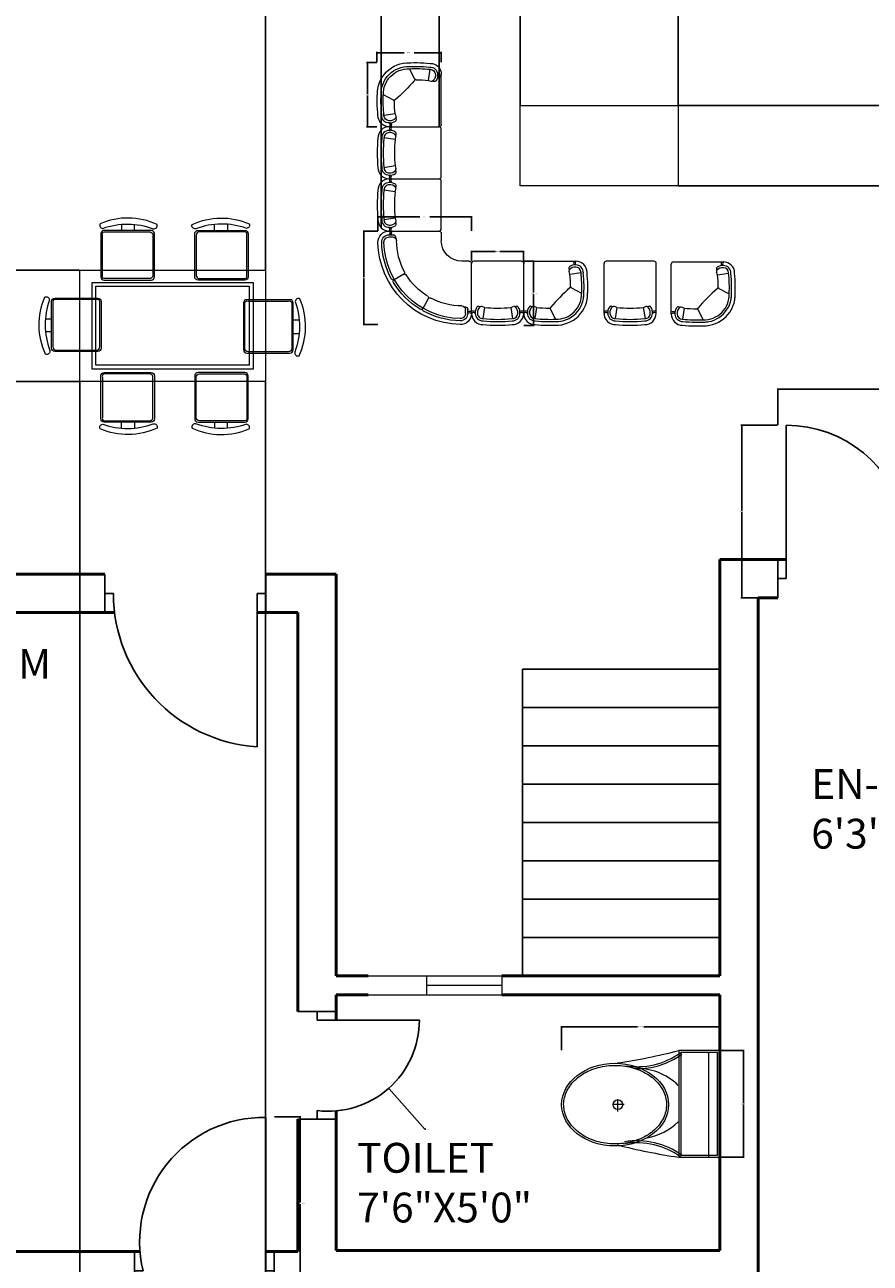
# Model space of a CAD drawing. Units: inches. Extents: x 2215 to 3724, y 1009 to 2124.
# Tile 3 of 11: x 2438 to 2636, y 1158 to 1449. Entities that reach past the tile are written whole.
import ezdxf

# ---------------------------------------------------------------- set-up
doc = ezdxf.new("R2010")
doc.units = ezdxf.units.IN
for name, color, linetype, lineweight in [('A-ANNO-DIMS', 2, 'Continuous', 18), ('A-AREA-IDEN', 7, 'Continuous', 18), ('A-DOOR', 3, 'Continuous', 25), ('A-FLOR-FIXT', 9, 'Continuous', 18), ('A-FLOR-STRS', 7, 'Continuous', 25), ('A-FURN', 8, 'Continuous', 18), ('A-GLAZ', 4, 'Continuous', 18), ('A-WALL', 7, 'Continuous', 50)]:
    doc.layers.add(name, color=color, linetype=linetype, lineweight=lineweight)
doc.styles.get("Standard").update_dxf_attribs({"font": 'arial.ttf'})
doc.dimstyles.get("Standard").update_dxf_attribs({"dimtxt": 0.18, "dimasz": 0.18, "dimexe": 0.18, "dimexo": 0.0625, "dimgap": 0.09, "dimtad": 0, "dimtih": 1, "dimtoh": 1, "dimdec": 4, "dimzin": 0, "dimdsep": 46, "dimtxsty": 'Standard', "dimcen": 0.09, "dimadec": 0, "dimazin": 0, "dimtfac": 1, "dimtdec": 4, "dimtofl": 0, "dimtmove": 0, "dimatfit": 3, "dimfxl": 1, "dimtolj": 1, "dimtzin": 0, "dimarcsym": 0})

# ---------------------------------------------------------------- blocks, each defined once
blk = doc.blocks.new('A$C31115884')
for p, q in [((283.1, 497.7), (223.4, 497.7)), ((257.5, 466.4), (257.5, 523.2)), ((0, 200), (0, 0)), ((520, 200), (0, 200)), ((10, 190), (10, 10)), ((510, 190), (10, 190)), ((510, 10), (510, 190)), ((520, 0), (520, 200)), ((510, 54.5), (0, 54.5)), ((10, 10), (510, 10)), ((0, 0), (520, 0))]:
    blk.add_line(p, q)
blk.add_circle((255.6, 496.4), 23.6)
for centre, radius, start, end in [((2777.7, -204.6), 2807, 165.4549, 171.71327), ((3237, 905), 2807, 188.28673, 194.5451), ((-294.5, 403.3), 364.7, 324.20913, 9.34987), ((-294.5, 403.3), 374.7, 324.20913, 9.34987), ((805.8, 403.3), 364.7, 170.65013, 215.79087), ((139.5, 406.2), 293.5, 315.84364, 2.65635), ((805.8, 403.3), 374.7, 179.20365, 215.79087), ((383.6, 406.2), 293.5, 190.27735, 224.15636)]:
    blk.add_arc(centre, radius, start, end)
blk.add_ellipse((256.2, 509.9), major_axis=(0, -260.7), ratio=0.772727)
blk.add_open_spline([(256.2, 259.2), (263.1, 259.2), (270, 259.7), (287.8, 262.3), (298.7, 265.1), (319.9, 273.1), (330.2, 278.4), (350.1, 291.1), (359.7, 298.7), (377.7, 315.9), (386.2, 325.5), (401.7, 346.6), (408.8, 358.1), (421.3, 382.5), (426.8, 395.5), (435.9, 422.4), (439.5, 436.4), (444.8, 465.1), (446.5, 479.7), (447.9, 509.2), (447.6, 524), (445, 553.3), (442.7, 567.8), (436.3, 596), (432.1, 609.7), (421.9, 636), (416, 648.6), (402.5, 672.1), (395, 683), (378.6, 703), (369.8, 712.1), (351.1, 728), (341.3, 734.8), (320.9, 746.2), (310.4, 750.7), (288.9, 757.3), (278, 759.4), (256, 761), (245, 760.6), (223.1, 757.2), (212.3, 754.3), (191.1, 746.1), (180.8, 740.7), (160.9, 727.8), (151.4, 720.1), (133.5, 702.7), (125.1, 693), (109.6, 671.7), (102.6, 660.2), (90.2, 635.7), (84.9, 622.7), (76, 595.6), (72.4, 581.6), (67.2, 552.9), (65.6, 538.2), (64.4, 508.8), (64.8, 494), (67.5, 464.7), (69.9, 450.2), (76.6, 422), (80.8, 408.3), (91.1, 382.2), (97.2, 369.7), (110.8, 346.3), (118.4, 335.4), (134.8, 315.6), (143.7, 306.7), (162.4, 290.9), (172.3, 284.2), (192.8, 273), (203.3, 268.6), (224.8, 262.2), (235.8, 260.2), (249.9, 259.3), (253, 259.2), (256.2, 259.2)], degree=3, knots=[0, 0, 0, 0, 0.110105, 0.110105, 0.285049, 0.285049, 0.459994, 0.459994, 0.634938, 0.634938, 0.809882, 0.809882, 0.984827, 0.984827, 1.159771, 1.159771, 1.334715, 1.334715, 1.50966, 1.50966, 1.684604, 1.684604, 1.859549, 1.859549, 2.034493, 2.034493, 2.209437, 2.209437, 2.384382, 2.384382, 2.559326, 2.559326, 2.73427, 2.73427, 2.909215, 2.909215, 3.084159, 3.084159, 3.259103, 3.259103, 3.434048, 3.434048, 3.608992, 3.608992, 3.783936, 3.783936, 3.958881, 3.958881, 4.133825, 4.133825, 4.30877, 4.30877, 4.483714, 4.483714, 4.658658, 4.658658, 4.833603, 4.833603, 5.008547, 5.008547, 5.183491, 5.183491, 5.358436, 5.358436, 5.53338, 5.53338, 5.708324, 5.708324, 5.883269, 5.883269, 6.058213, 6.058213, 6.233158, 6.233158, 6.283185, 6.283185, 6.283185, 6.283185])
blk = doc.blocks.new('A$C707258B2')
at = {"color": 0}
for p, q in [((0.404, 0.342), (1.074, 0.342)), ((0.404, 0.292), (0.454, 0.292)), ((0.404, 0.262), (0.454, 0.262)), ((1.104, 0.312), (1.104, 0.212)), ((1.479, -0.063), (1.379, -0.063)), ((1.509, -0.763), (1.509, -0.093)), ((0.6, -0.238), (0.47, -0.313)), ((0.929, -0.567), (0.854, -0.697)), ((1.429, -0.763), (1.429, -0.713)), ((1.459, -0.763), (1.459, -0.712))]:
    blk.add_line(p, q, dxfattribs=at)
for centre, radius, start, end in [((0.404, 0.192), 0.15, 90, 181.1754), ((0.378, 0.317), 0.0362, 316.3972, 43.6028), ((0.368, 0.317), 0.0662, 337.8298, 22.1702), ((1.074, 0.312), 0.03, 360, 90), ((1.379, 0.212), 1.125, 181.1754, 268.8246), ((0.404, 0.192), 0.1, 90, 181.1754), ((1.379, 0.212), 1.075, 181.1754, 208.6357), ((0.404, 0.192), 0.07, 90, 181.1754), ((1.379, 0.212), 1.045, 181.1754, 268.8246), ((0.455, 0.256), 0.0357, 345.4262, 90.5555), ((0.454, 0.212), 0.05, 360, 90), ((1.379, 0.212), 0.875, 180, 208.4082), ((1.379, 0.212), 0.275, 180, 270), ((1.479, -0.093), 0.03, 360, 90), ((0.457, -0.291), 0.025, 208.6357, 300), ((0.482, -0.334), 0.025, 120, 211.3643), ((0.587, -0.216), 0.025, 300, 28.4082), ((0.612, -0.259), 0.025, 31.5918, 120), ((1.379, 0.212), 0.875, 211.5918, 238.4082), ((1.379, 0.212), 1.075, 211.3643, 238.6357), ((0.907, -0.555), 0.025, 330, 58.4082), ((0.951, -0.58), 0.025, 61.5918, 150), ((1.379, 0.212), 0.875, 241.5918, 270), ((1.379, -0.713), 0.05, 360, 90), ((0.832, -0.685), 0.025, 238.6357, 330), ((0.876, -0.71), 0.025, 150, 241.3643), ((1.379, 0.212), 1.075, 241.3643, 268.8246), ((1.359, -0.763), 0.15, 268.8246, 360), ((1.359, -0.763), 0.1, 268.8246, 360), ((1.359, -0.763), 0.07, 268.8246, 360), ((1.425, -0.709), 0.0336, 354.6301, 109.3883), ((1.484, -0.799), 0.0662, 67.8298, 112.1702), ((1.484, -0.789), 0.0362, 46.3972, 133.6028)]:
    blk.add_arc(centre, radius, start, end, dxfattribs=at)
blk = doc.blocks.new('part 01')
at = {"color": 0}
for p, q in [((-670, 700), (0, 700)), ((30, 30), (30, 670)), ((-591, 527), (-740, 550)), ((-591, 527), (-579, 561)), ((-591, 173), (-740, 150)), ((-591, 173), (-579, 139)), ((-670, 0), (0, 0))]:
    blk.add_line(p, q, dxfattribs=at)
for centre, radius, start, end in [((-670, 550), 150, 90, 181.1754), ((-696, 675), 36.2, 316.3972, 43.6028), ((-706, 675), 66.2, 337.8298, 22.1702), ((0, 670), 30, 0, 90), ((1178, 350), 2008, 174.2835, 185.7165), ((1178, 350), 1958, 174.2835, 185.7165), ((-670, 550), 100, 90, 181.1754), ((1178, 350), 1928, 174.2835, 185.7165), ((-670, 550), 70, 90, 181.1754), ((-660, 518), 133, 56.0897, 95.6132), ((-660, 518), 103, 42.0066, 95.6132), ((1178, 350), 1778, 174.2835, 185.7165), ((-600, 607), 25, 332.9608, 56.0897), ((-625, 620), 53.2, 321.0017, 332.9608), ((-602, 570), 25, 340, 42.0066), ((-670, 150), 150, 178.8246, 270), ((-670, 150), 100, 178.8246, 270), ((-670, 150), 70, 178.8246, 270), ((-660, 182), 133, 264.3868, 303.9103), ((-660, 182), 103, 264.3868, 317.9934), ((-696, 25), 36.2, 316.3972, 43.6028), ((-706, 25), 66.2, 337.8298, 22.1702), ((-600, 93), 25, 303.9103, 27.0392), ((-602, 130), 25, 317.9934, 20), ((-625, 80), 53.2, 27.0392, 38.9983), ((0, 30), 30, 270, 0)]:
    blk.add_arc(centre, radius, start, end, dxfattribs=at)
blk = doc.blocks.new('part02')
at = {"color": 0}
for p, q in [((0, -670), (0, 0)), ((30, 30), (700, 30)), ((621, -143), (609, -109)), ((621, -143), (770, -120)), ((640, -326), (778, -399)), ((173, -591), (139, -579)), ((173, -591), (150, -740)), ((356, -610), (429, -748))]:
    blk.add_line(p, q, dxfattribs=at)
for centre, radius, start, end in [((30, 0), 30, 90, 180), ((726, 5), 56.2, 153.6122, 206.6666), ((726, 5), 36.2, 136.3972, 223.6028), ((700, -120), 150, 0, 90), ((630, -63), 25, 123.9103, 207.0392), ((655, -50), 53.2, 207.0392, 218.9983), ((632, -100), 25, 137.9934, 200), ((690, -152), 103, 84.3868, 137.9934), ((689, -151), 132, 85.4378, 123.9887), ((-1148, -320), 1778, 0.3836, 5.7165), ((700, -121), 101, 357.5006, 89.858), ((700, -120), 70, 0, 90), ((-1228, -320), 2008, 357.7349, 5.7032), ((-1148, -320), 1958, 355.8657, 5.7165), ((-1148, -320), 2008, 355.818, 5.7165), ((2220, -2190), 2454, 130.6961, 139.3039), ((632, -344), 20, 62, 130.6961), ((650, -308), 20, 180.3836, 242), ((439, -409), 419, 268.2181, 1.7819), ((439, -409), 369, 268.2181, 1.7819), ((439, -409), 339, 268.2181, 1.7819), ((25, -696), 56.2, 63.3334, 116.3878), ((25, -696), 36.2, 46.3972, 133.6028), ((182, -660), 133, 146.0897, 185.6132), ((93, -600), 25, 62.9608, 146.0897), ((182, -660), 103, 132.0066, 185.6132), ((80, -625), 53.2, 51.0017, 62.9608), ((130, -602), 25, 70, 132.0066), ((350, 1178), 1778, 264.2835, 269.6164), ((338, -620), 20, 28, 89.6164), ((374, -602), 20, 139.3039, 208), ((150, -670), 150, 180, 271.1754), ((150, -670), 100, 180, 271.1754), ((150, -670), 70, 180, 270), ((350, 1258), 2008, 264.2968, 272.2651), ((350, 1178), 2008, 264.2835, 274.182), ((350, 1178), 1958, 264.2835, 274.1343)]:
    blk.add_arc(centre, radius, start, end, dxfattribs=at)
blk = doc.blocks.new('DOOR-ENTRY-PAIR')
for p, q in [((2, 4.5), (2, 40.5)), ((54.26, 4.5), (54.26, 40.5)), ((0, 9), (0, 0)), ((56.26, 9), (56.26, 0)), ((0, 0), (0, 4.5)), ((0, 4.5), (2, 4.5)), ((56.26, 4.5), (54.26, 4.5))]:
    blk.add_line(p, q)
for centre, radius, start, end in [((2, 12.02), 28.48, 11.0167, 90), ((55.55, 14.8), 25.73, 92.8796, 174.0708)]:
    blk.add_arc(centre, radius, start, end)
blk = doc.blocks.new('DOOR-FRONT-SINGLE')
for p, q in [((30.79, 4.5), (30.79, 40.5)), ((0, 9), (0, 0)), ((32.79, 9), (32.79, 0)), ((0, 0), (0, 4.5)), ((0, 4.5), (2, 4.5)), ((32.79, 4.5), (30.79, 4.5)), ((32.79, 0), (32.79, 4.5))]:
    blk.add_line(p, q)
blk.add_arc((30.39, 11.3), 29.2, 89.2162, 193.4744)
blk = doc.blocks.new('DOOR-DRAWING-ROOM')
for p, q in [((0, 40.5), (0, 31.5)), ((37.77, 40.5), (37.77, 31.5)), ((0, 31.5), (0, 36)), ((0, 36), (2, 36)), ((37.77, 36), (35.77, 36)), ((35.77, 36), (35.77, 0)), ((37.77, 31.5), (37.77, 36))]:
    blk.add_line(p, q)
blk.add_arc((38.07, 36), 36.07, 180, 266.3399)
blk = doc.blocks.new('DOOR-BATH-FRONT')
for p, q in [((9, 25.25), (0, 25.25)), ((0, 25.25), (4.5, 25.25)), ((4.5, 25.25), (4.5, 23.25)), ((4.5, 23.25), (28.5, 23.25)), ((4.5, 0), (4.5, 2)), ((0, 0), (9, 0)), ((9, 0), (4.5, 0))]:
    blk.add_line(p, q)
blk.add_arc((7.1, 23.25), 21.4, 263.0342, 0)
blk = doc.blocks.new('VENT-FRONT-BATH')
for p, q in [((0, 4.5), (31.33, 4.5)), ((13.67, 4.5), (13.67, 4.5)), ((13.67, 4.5), (13.67, 0)), ((31.33, 4.5), (31.33, 0)), ((31.33, 2.25), (13.67, 2.25)), ((0, 0), (0, 0)), ((0, 0), (0, 0)), ((0, 0), (31.33, 0))]:
    blk.add_line(p, q)
blk = doc.blocks.new('STAIR-FLIGHT-PLAN')
for p, q in [((0, 0), (0, 72)), ((46.33, 72), (0, 72)), ((46.33, 63), (0, 63)), ((46.33, 54), (0, 54)), ((46.33, 45), (0, 45)), ((46.33, 36), (0, 36)), ((46.33, 27), (0, 27)), ((46.33, 18), (0, 18)), ((46.33, 9), (0, 9))]:
    blk.add_line(p, q)
blk = doc.blocks.new('*D57')
at = {"layer": 'A-ANNO-DIMS', "color": 0, "lineweight": -2, "transparency": 16777216}
for p, q in [((2614.45, 1355.05), (2614.45, 1363.61)), ((2670.71, 1355.05), (2670.71, 1363.61)), ((2614.63, 1363.43), (2641.27, 1363.43)), ((2670.53, 1363.43), (2643.9, 1363.43))]:
    blk.add_line(p, q, dxfattribs=at)
at = {"layer": 'A-ANNO-DIMS', "color": 0, "transparency": 16777216}
for points in [[(2614.63, 1363.46), (2614.63, 1363.4), (2614.45, 1363.43)], [(2670.53, 1363.46), (2670.53, 1363.4), (2670.71, 1363.43)]]:
    blk.add_solid(points, dxfattribs=at)
at = {"layer": 'Defpoints', "color": 0, "transparency": 16777216}
for p in [(2670.71, 1363.43), (2614.45, 1354.99), (2670.71, 1354.99)]:
    blk.add_point(p, dxfattribs=at)
at = {"layer": 'A-ANNO-DIMS', "color": 0, "transparency": 16777216, "insert": (2642.58, 1363.43), "char_height": 0.18, "attachment_point": 5}
blk.add_mtext('\\A1;ENTRY PAIR 56 TYP.', dxfattribs=at)
blk = doc.blocks.new('*D58')
at = {"layer": 'A-ANNO-DIMS', "color": 0, "lineweight": -2, "transparency": 16777216}
for p, q in [((2614.39, 1354.99), (2605.83, 1354.99)), ((2606.01, 1354.81), (2606.01, 1334.92)), ((2606.01, 1314.67), (2606.01, 1334.56)), ((2614.39, 1314.49), (2605.83, 1314.49))]:
    blk.add_line(p, q, dxfattribs=at)
at = {"layer": 'A-ANNO-DIMS', "color": 0, "transparency": 16777216}
for points in [[(2605.98, 1354.81), (2606.04, 1354.81), (2606.01, 1354.99)], [(2605.98, 1314.67), (2606.04, 1314.67), (2606.01, 1314.49)]]:
    blk.add_solid(points, dxfattribs=at)
at = {"layer": 'Defpoints', "color": 0, "transparency": 16777216}
for p in [(2606.01, 1354.99), (2614.45, 1354.99), (2614.45, 1314.49)]:
    blk.add_point(p, dxfattribs=at)
at = {"layer": 'A-ANNO-DIMS', "color": 0, "transparency": 16777216, "insert": (2606.01, 1334.74), "char_height": 0.18, "attachment_point": 5}
blk.add_mtext('\\A1;41 TYP.', dxfattribs=at)
blk = doc.blocks.new('*D67')
at = {"layer": 'A-ANNO-DIMS', "color": 0, "lineweight": -2, "transparency": 16777216}
for p, q in [((2496.34, 1192.62), (2502.55, 1192.62)), ((2502.37, 1192.44), (2502.37, 1172.49)), ((2502.37, 1152.18), (2502.37, 1172.13)), ((2496.34, 1152), (2502.55, 1152))]:
    blk.add_line(p, q, dxfattribs=at)
at = {"layer": 'A-ANNO-DIMS', "color": 0, "transparency": 16777216}
for points in [[(2502.34, 1192.44), (2502.4, 1192.44), (2502.37, 1192.62)], [(2502.34, 1152.18), (2502.4, 1152.18), (2502.37, 1152)]]:
    blk.add_solid(points, dxfattribs=at)
at = {"layer": 'Defpoints', "color": 0, "transparency": 16777216}
for p in [(2496.28, 1192.62), (2502.37, 1192.62), (2496.28, 1152)]:
    blk.add_point(p, dxfattribs=at)
at = {"layer": 'A-ANNO-DIMS', "color": 0, "transparency": 16777216, "insert": (2502.37, 1172.31), "char_height": 0.18, "attachment_point": 5}
blk.add_mtext('\\A1;ENTRY DOOR 41 TYP.', dxfattribs=at)
blk = doc.blocks.new('*D79')
at = {"layer": 'A-ANNO-DIMS', "color": 0, "lineweight": -2, "transparency": 16777216}
for p, q in [((2563.73, 1208.26), (2563.73, 1213.95)), ((2563.91, 1213.77), (2581.51, 1213.77)), ((2600.66, 1213.77), (2583.06, 1213.77)), ((2600.84, 1208.26), (2600.84, 1213.95))]:
    blk.add_line(p, q, dxfattribs=at)
at = {"layer": 'A-ANNO-DIMS', "color": 0, "transparency": 16777216}
for points in [[(2563.91, 1213.8), (2563.91, 1213.74), (2563.73, 1213.77)], [(2600.66, 1213.8), (2600.66, 1213.74), (2600.84, 1213.77)]]:
    blk.add_solid(points, dxfattribs=at)
at = {"layer": 'Defpoints', "color": 0, "transparency": 16777216}
for p in [(2563.73, 1213.77), (2563.73, 1208.2), (2600.84, 1208.2)]:
    blk.add_point(p, dxfattribs=at)
at = {"layer": 'A-ANNO-DIMS', "color": 0, "transparency": 16777216, "insert": (2582.28, 1213.77), "char_height": 0.18, "attachment_point": 5}
blk.add_mtext('\\A1;WC 37 TYP.', dxfattribs=at)
blk = doc.blocks.new('*D80')
at = {"layer": 'A-ANNO-DIMS', "color": 0, "lineweight": -2, "transparency": 16777216}
for p, q in [((2600.9, 1208.2), (2606.59, 1208.2)), ((2606.41, 1208.02), (2606.41, 1195.86)), ((2606.41, 1183.33), (2606.41, 1195.5)), ((2600.9, 1183.15), (2606.59, 1183.15))]:
    blk.add_line(p, q, dxfattribs=at)
at = {"layer": 'A-ANNO-DIMS', "color": 0, "transparency": 16777216}
for points in [[(2606.38, 1208.02), (2606.44, 1208.02), (2606.41, 1208.2)], [(2606.38, 1183.33), (2606.44, 1183.33), (2606.41, 1183.15)]]:
    blk.add_solid(points, dxfattribs=at)
at = {"layer": 'Defpoints', "color": 0, "transparency": 16777216}
for p in [(2600.84, 1208.2), (2606.41, 1208.2), (2600.84, 1183.15)]:
    blk.add_point(p, dxfattribs=at)
at = {"layer": 'A-ANNO-DIMS', "color": 0, "transparency": 16777216, "insert": (2606.41, 1195.68), "char_height": 0.18, "attachment_point": 5}
blk.add_mtext('\\A1;25 TYP.', dxfattribs=at)
blk = doc.blocks.new('*D81')
at = {"layer": 'A-ANNO-DIMS', "color": 0, "lineweight": -2, "transparency": 16777216}
for p, q in [((2554.88, 1393.49), (2557.27, 1393.49)), ((2557.09, 1393.31), (2557.09, 1386.12)), ((2557.09, 1378.57), (2557.09, 1385.76)), ((2554.88, 1378.39), (2557.27, 1378.39))]:
    blk.add_line(p, q, dxfattribs=at)
at = {"layer": 'A-ANNO-DIMS', "color": 0, "transparency": 16777216}
for points in [[(2557.06, 1393.31), (2557.12, 1393.31), (2557.09, 1393.49)], [(2557.06, 1378.57), (2557.12, 1378.57), (2557.09, 1378.39)]]:
    blk.add_solid(points, dxfattribs=at)
at = {"layer": 'Defpoints', "color": 0, "transparency": 16777216}
for p in [(2554.82, 1393.49), (2557.09, 1393.49), (2554.82, 1378.39)]:
    blk.add_point(p, dxfattribs=at)
at = {"layer": 'A-ANNO-DIMS', "color": 0, "transparency": 16777216, "insert": (2557.09, 1385.94), "char_height": 0.18, "attachment_point": 5}
blk.add_mtext('\\A1;SOFA SEAT 15 TYP.', dxfattribs=at)
blk = doc.blocks.new('*D82')
at = {"layer": 'A-ANNO-DIMS', "color": 0, "lineweight": -2, "transparency": 16777216}
for p, q in [((2542.57, 1393.55), (2542.57, 1395.94)), ((2542.75, 1395.76), (2548.18, 1395.76)), ((2554.64, 1395.76), (2549.22, 1395.76)), ((2554.82, 1393.55), (2554.82, 1395.94))]:
    blk.add_line(p, q, dxfattribs=at)
at = {"layer": 'A-ANNO-DIMS', "color": 0, "transparency": 16777216}
for points in [[(2542.75, 1395.79), (2542.75, 1395.73), (2542.57, 1395.76)], [(2554.64, 1395.79), (2554.64, 1395.73), (2554.82, 1395.76)]]:
    blk.add_solid(points, dxfattribs=at)
at = {"layer": 'Defpoints', "color": 0, "transparency": 16777216}
for p in [(2542.57, 1395.76), (2542.57, 1393.49), (2554.82, 1393.49)]:
    blk.add_point(p, dxfattribs=at)
at = {"layer": 'A-ANNO-DIMS', "color": 0, "transparency": 16777216, "insert": (2548.7, 1395.76), "char_height": 0.18, "attachment_point": 5}
blk.add_mtext('\\A1;12 TYP.', dxfattribs=at)
blk = doc.blocks.new('*D83')
at = {"layer": 'A-ANNO-DIMS', "color": 0, "lineweight": -2, "transparency": 16777216}
for p, q in [((2520.39, 1440.23), (2520.39, 1442.61)), ((2520.57, 1442.43), (2526.74, 1442.43)), ((2535.31, 1442.43), (2529.15, 1442.43)), ((2535.49, 1440.23), (2535.49, 1442.61))]:
    blk.add_line(p, q, dxfattribs=at)
at = {"layer": 'A-ANNO-DIMS', "color": 0, "transparency": 16777216}
for points in [[(2520.57, 1442.46), (2520.57, 1442.4), (2520.39, 1442.43)], [(2535.31, 1442.46), (2535.31, 1442.4), (2535.49, 1442.43)]]:
    blk.add_solid(points, dxfattribs=at)
at = {"layer": 'Defpoints', "color": 0, "transparency": 16777216}
for p in [(2535.49, 1442.43), (2520.39, 1440.16), (2535.49, 1440.16)]:
    blk.add_point(p, dxfattribs=at)
at = {"layer": 'A-ANNO-DIMS', "color": 0, "transparency": 16777216, "insert": (2527.94, 1442.43), "char_height": 0.18, "attachment_point": 5}
blk.add_mtext('\\A1;SOFA END 15 TYP.', dxfattribs=at)
blk = doc.blocks.new('*D84')
at = {"layer": 'A-ANNO-DIMS', "color": 0, "lineweight": -2, "transparency": 16777216}
for p, q in [((2520.33, 1440.16), (2517.95, 1440.16)), ((2518.13, 1439.98), (2518.13, 1432.8)), ((2518.13, 1425.25), (2518.13, 1432.43)), ((2520.33, 1425.07), (2517.95, 1425.07))]:
    blk.add_line(p, q, dxfattribs=at)
at = {"layer": 'A-ANNO-DIMS', "color": 0, "transparency": 16777216}
for points in [[(2518.1, 1439.98), (2518.16, 1439.98), (2518.13, 1440.16)], [(2518.1, 1425.25), (2518.16, 1425.25), (2518.13, 1425.07)]]:
    blk.add_solid(points, dxfattribs=at)
at = {"layer": 'Defpoints', "color": 0, "transparency": 16777216}
for p in [(2518.13, 1440.16), (2520.39, 1440.16), (2520.39, 1425.07)]:
    blk.add_point(p, dxfattribs=at)
at = {"layer": 'A-ANNO-DIMS', "color": 0, "transparency": 16777216, "insert": (2518.13, 1432.62), "char_height": 0.18, "attachment_point": 5}
blk.add_mtext('\\A1;15 TYP.', dxfattribs=at)
blk = doc.blocks.new('*D85')
at = {"layer": 'A-ANNO-DIMS', "color": 0, "lineweight": -2, "transparency": 16777216}
for p, q in [((2520.61, 1400.64), (2520.61, 1404.05)), ((2520.79, 1403.87), (2530.42, 1403.87)), ((2542.39, 1403.87), (2532.77, 1403.87)), ((2542.57, 1400.64), (2542.57, 1404.05))]:
    blk.add_line(p, q, dxfattribs=at)
at = {"layer": 'A-ANNO-DIMS', "color": 0, "transparency": 16777216}
for points in [[(2520.79, 1403.9), (2520.79, 1403.84), (2520.61, 1403.87)], [(2542.39, 1403.9), (2542.39, 1403.84), (2542.57, 1403.87)]]:
    blk.add_solid(points, dxfattribs=at)
at = {"layer": 'Defpoints', "color": 0, "transparency": 16777216}
for p in [(2542.57, 1403.87), (2520.61, 1400.58), (2542.57, 1400.58)]:
    blk.add_point(p, dxfattribs=at)
at = {"layer": 'A-ANNO-DIMS', "color": 0, "transparency": 16777216, "insert": (2531.59, 1403.87), "char_height": 0.18, "attachment_point": 5}
blk.add_mtext('\\A1;SOFA CORNER 22', dxfattribs=at)
blk = doc.blocks.new('*D86')
at = {"layer": 'A-ANNO-DIMS', "color": 0, "lineweight": -2, "transparency": 16777216}
for p, q in [((2520.55, 1400.58), (2517.13, 1400.58)), ((2517.31, 1400.4), (2517.31, 1389.77)), ((2517.31, 1378.79), (2517.31, 1389.41)), ((2520.55, 1378.61), (2517.13, 1378.61))]:
    blk.add_line(p, q, dxfattribs=at)
at = {"layer": 'A-ANNO-DIMS', "color": 0, "transparency": 16777216}
for points in [[(2517.28, 1400.4), (2517.34, 1400.4), (2517.31, 1400.58)], [(2517.28, 1378.79), (2517.34, 1378.79), (2517.31, 1378.61)]]:
    blk.add_solid(points, dxfattribs=at)
at = {"layer": 'Defpoints', "color": 0, "transparency": 16777216}
for p in [(2517.31, 1400.58), (2520.61, 1400.58), (2520.61, 1378.61)]:
    blk.add_point(p, dxfattribs=at)
at = {"layer": 'A-ANNO-DIMS', "color": 0, "transparency": 16777216, "insert": (2517.31, 1389.59), "char_height": 0.18, "attachment_point": 5}
blk.add_mtext('\\A1;22', dxfattribs=at)
blk = doc.blocks.new('*D99')
at = {"layer": 'A-ANNO-DIMS', "color": 0, "lineweight": -2, "transparency": 16777216}
for p, q in [((2684.84, 1343.93), (2684.84, 1118.22)), ((2609.84, 1151.93), (2609.84, 1118.22)), ((2610.02, 1118.4), (2647.12, 1118.4)), ((2684.66, 1118.4), (2647.56, 1118.4))]:
    blk.add_line(p, q, dxfattribs=at)
at = {"layer": 'A-ANNO-DIMS', "color": 0, "transparency": 16777216}
for points in [[(2610.02, 1118.43), (2610.02, 1118.37), (2609.84, 1118.4)], [(2684.66, 1118.43), (2684.66, 1118.37), (2684.84, 1118.4)]]:
    blk.add_solid(points, dxfattribs=at)
at = {"layer": 'Defpoints', "color": 0, "transparency": 16777216}
for p in [(2684.84, 1344), (2609.84, 1152), (2684.84, 1118.4)]:
    blk.add_point(p, dxfattribs=at)
at = {"layer": 'A-ANNO-DIMS', "color": 0, "transparency": 16777216, "insert": (2647.34, 1118.4), "char_height": 0.18, "attachment_point": 5}
blk.add_mtext('\\A1;75', dxfattribs=at)
blk = doc.blocks.new('*D102')
at = {"layer": 'A-ANNO-DIMS', "color": 0, "lineweight": -2, "transparency": 16777216}
for p, q in [((2450.62, 1365.21), (2450.62, 1118.22)), ((2494.2, 1365.21), (2494.2, 1118.22)), ((2450.8, 1118.4), (2472.01, 1118.4)), ((2494.02, 1118.4), (2472.8, 1118.4))]:
    blk.add_line(p, q, dxfattribs=at)
at = {"layer": 'A-ANNO-DIMS', "color": 0, "transparency": 16777216}
for points in [[(2450.8, 1118.43), (2450.8, 1118.37), (2450.62, 1118.4)], [(2494.02, 1118.43), (2494.02, 1118.37), (2494.2, 1118.4)]]:
    blk.add_solid(points, dxfattribs=at)
at = {"layer": 'Defpoints', "color": 0, "transparency": 16777216}
for p in [(2450.62, 1365.28), (2494.2, 1365.28), (2494.2, 1118.4)]:
    blk.add_point(p, dxfattribs=at)
at = {"layer": 'A-ANNO-DIMS', "color": 0, "transparency": 16777216, "insert": (2472.41, 1118.4), "char_height": 0.18, "attachment_point": 5}
blk.add_mtext('\\A1;43.58', dxfattribs=at)
blk = doc.blocks.new('*D103')
at = {"layer": 'A-ANNO-DIMS', "color": 0, "lineweight": -2, "transparency": 16777216}
for p, q in [((2450.55, 1391.42), (2279.06, 1391.42)), ((2279.24, 1391.24), (2279.24, 1378.53)), ((2279.24, 1365.46), (2279.24, 1378.17)), ((2450.55, 1365.28), (2279.06, 1365.28))]:
    blk.add_line(p, q, dxfattribs=at)
at = {"layer": 'A-ANNO-DIMS', "color": 0, "transparency": 16777216}
for points in [[(2279.21, 1391.24), (2279.27, 1391.24), (2279.24, 1391.42)], [(2279.21, 1365.46), (2279.27, 1365.46), (2279.24, 1365.28)]]:
    blk.add_solid(points, dxfattribs=at)
at = {"layer": 'Defpoints', "color": 0, "transparency": 16777216}
for p in [(2279.24, 1391.42), (2450.62, 1391.42), (2450.62, 1365.28)]:
    blk.add_point(p, dxfattribs=at)
at = {"layer": 'A-ANNO-DIMS', "color": 0, "transparency": 16777216, "insert": (2279.24, 1378.35), "char_height": 0.18, "attachment_point": 5}
blk.add_mtext('\\A1;26.147', dxfattribs=at)
blk = doc.blocks.new('*D104')
at = {"layer": 'A-ANNO-DIMS', "color": 0, "lineweight": -2, "transparency": 16777216}
for p, q in [((2553.99, 1430.08), (2553.99, 1781.28)), ((2554.17, 1781.1), (2572.13, 1781.1)), ((2590.88, 1781.1), (2572.92, 1781.1)), ((2591.06, 1430.08), (2591.06, 1781.28))]:
    blk.add_line(p, q, dxfattribs=at)
at = {"layer": 'A-ANNO-DIMS', "color": 0, "transparency": 16777216}
for points in [[(2554.17, 1781.13), (2554.17, 1781.07), (2553.99, 1781.1)], [(2590.88, 1781.13), (2590.88, 1781.07), (2591.06, 1781.1)]]:
    blk.add_solid(points, dxfattribs=at)
at = {"layer": 'Defpoints', "color": 0, "transparency": 16777216}
for p in [(2591.06, 1781.1), (2553.99, 1430.02), (2591.06, 1430.02)]:
    blk.add_point(p, dxfattribs=at)
at = {"layer": 'A-ANNO-DIMS', "color": 0, "transparency": 16777216, "insert": (2572.53, 1781.1), "char_height": 0.18, "attachment_point": 5}
blk.add_mtext('\\A1;37.07', dxfattribs=at)
blk = doc.blocks.new('*D105')
at = {"layer": 'A-ANNO-DIMS', "color": 0, "lineweight": -2, "transparency": 16777216}
for p, q in [((2591.12, 1430.02), (2904.62, 1430.02)), ((2904.44, 1429.84), (2904.44, 1420.79)), ((2904.44, 1411.39), (2904.44, 1420.43)), ((2591.12, 1411.21), (2904.62, 1411.21))]:
    blk.add_line(p, q, dxfattribs=at)
at = {"layer": 'A-ANNO-DIMS', "color": 0, "transparency": 16777216}
for points in [[(2904.41, 1429.84), (2904.47, 1429.84), (2904.44, 1430.02)], [(2904.41, 1411.39), (2904.47, 1411.39), (2904.44, 1411.21)]]:
    blk.add_solid(points, dxfattribs=at)
at = {"layer": 'Defpoints', "color": 0, "transparency": 16777216}
for p in [(2591.06, 1430.02), (2904.44, 1430.02), (2591.06, 1411.21)]:
    blk.add_point(p, dxfattribs=at)
at = {"layer": 'A-ANNO-DIMS', "color": 0, "transparency": 16777216, "insert": (2904.44, 1420.61), "char_height": 0.18, "attachment_point": 5}
blk.add_mtext('\\A1;18.81', dxfattribs=at)
blk = doc.blocks.new('*D106')
at = {"layer": 'A-ANNO-DIMS', "color": 0, "lineweight": -2, "transparency": 16777216}
for p, q in [((2494.2, 1391.49), (2494.2, 1781.28)), ((2494.38, 1781.1), (2507.39, 1781.1)), ((2521.19, 1781.1), (2508.18, 1781.1)), ((2521.37, 1401.43), (2521.37, 1781.28))]:
    blk.add_line(p, q, dxfattribs=at)
at = {"layer": 'A-ANNO-DIMS', "color": 0, "transparency": 16777216}
for points in [[(2494.38, 1781.13), (2494.38, 1781.07), (2494.2, 1781.1)], [(2521.19, 1781.13), (2521.19, 1781.07), (2521.37, 1781.1)]]:
    blk.add_solid(points, dxfattribs=at)
at = {"layer": 'Defpoints', "color": 0, "transparency": 16777216}
for p in [(2521.37, 1781.1), (2521.37, 1401.36), (2494.2, 1391.42)]:
    blk.add_point(p, dxfattribs=at)
at = {"layer": 'A-ANNO-DIMS', "color": 0, "transparency": 16777216, "insert": (2507.78, 1781.1), "char_height": 0.18, "attachment_point": 5}
blk.add_mtext('\\A1;27.18', dxfattribs=at)
blk = doc.blocks.new('*D107')
at = {"layer": 'A-ANNO-DIMS', "color": 0, "lineweight": -2, "transparency": 16777216}
for p, q in [((2534.96, 1425.13), (2534.96, 1781.28)), ((2535.14, 1781.1), (2544.02, 1781.1)), ((2553.81, 1781.1), (2544.93, 1781.1)), ((2553.99, 1430.08), (2553.99, 1781.28))]:
    blk.add_line(p, q, dxfattribs=at)
at = {"layer": 'A-ANNO-DIMS', "color": 0, "transparency": 16777216}
for points in [[(2535.14, 1781.13), (2535.14, 1781.07), (2534.96, 1781.1)], [(2553.81, 1781.13), (2553.81, 1781.07), (2553.99, 1781.1)]]:
    blk.add_solid(points, dxfattribs=at)
at = {"layer": 'Defpoints', "color": 0, "transparency": 16777216}
for p in [(2553.99, 1781.1), (2553.99, 1430.02), (2534.96, 1425.07)]:
    blk.add_point(p, dxfattribs=at)
at = {"layer": 'A-ANNO-DIMS', "color": 0, "transparency": 16777216, "insert": (2544.48, 1781.1), "char_height": 0.18, "attachment_point": 5}
blk.add_mtext('\\A1;19.027', dxfattribs=at)
blk = doc.blocks.new('*D139')
at = {"layer": 'A-ANNO-DIMS', "color": 0, "lineweight": -2, "transparency": 16777216}
for p, q in [((2508.85, 1215.34), (2509.03, 1215.34)), ((2508.94, 1215.25), (2508.94, 1215.43)), ((2531.64, 1189.7), (2523.25, 1199.18)), ((2531.82, 1189.7), (2531.64, 1189.7))]:
    blk.add_line(p, q, dxfattribs=at)
at = {"layer": 'A-ANNO-DIMS', "color": 0, "transparency": 16777216}
blk.add_solid([(2523.27, 1199.2), (2523.22, 1199.16), (2523.13, 1199.31)], dxfattribs=at)
at = {"layer": 'Defpoints', "color": 0, "transparency": 16777216}
for p in [(2508.94, 1215.34), (2523.13, 1199.31)]:
    blk.add_point(p, dxfattribs=at)
at = {"layer": 'A-ANNO-DIMS', "color": 0, "transparency": 16777216, "insert": (2532.37, 1189.7), "char_height": 0.18, "attachment_point": 5}
blk.add_mtext('\\A1;R21.404', dxfattribs=at)

msp = doc.modelspace()

# ---------------------------------------------------------------- linework, layer by layer
at = {"layer": 'A-FURN'}
for points in [[(2553.9914, 1430.018), (2591.0617, 1430.018), (2591.0617, 1411.2079), (2553.9914, 1411.2079)], [(2450.6169, 1391.4229), (2494.1952, 1391.4229), (2494.1952, 1365.276), (2450.6169, 1365.276)], [(2453.5221, 1388.5177), (2491.29, 1388.5177), (2491.29, 1368.1812), (2453.5221, 1368.1812)], [(2454.3937, 1387.6462), (2490.4184, 1387.6462), (2490.4184, 1369.0527), (2454.3937, 1369.0527)]]:
    msp.add_lwpolyline(points, close=True, dxfattribs=at)
for points in [[(2456.0071, 1401.2054, -0.17580919), (2467.8766, 1401.1155, 0.57839206), (2468.7758, 1402.1042, 0.21452438), (2455.3776, 1402.284, 0.55201397), (2456.0071, 1401.2053, -0.06507904)], [(2463.5025, 1400.729), (2463.5025, 1402.1226, -0.06475861)], [(2477.8691, 1401.1155, -0.57839206), (2476.9699, 1402.1042, -0.21452438), (2490.3681, 1402.284, -0.55201397), (2489.7386, 1401.2053, 0.1758092), (2477.8692, 1401.1155)], [(2482.2432, 1400.729), (2482.2432, 1402.1226, 0.06475861)], [(2467.373, 1400.729), (2456.3538, 1400.729, 0.41421356), (2455.5828, 1399.958), (2455.5828, 1389.8261, 0.41421356), (2456.3538, 1389.0552), (2467.373, 1389.0552, 0.41421356), (2468.1439, 1389.8261), (2468.1439, 1399.958, 0.41421356), (2467.373, 1400.729)], [(2489.392, 1400.729, -0.41421356), (2490.1629, 1399.958), (2490.1629, 1389.8261, -0.41421356), (2489.392, 1389.0552), (2478.3727, 1389.0552, -0.41421356), (2477.6018, 1389.8261), (2477.6018, 1399.958, -0.41421356), (2478.3727, 1400.729), (2489.392, 1400.729)], [(2443.5893, 1372.5423, -0.57839206), (2442.6006, 1371.6431, -0.21452438), (2442.4208, 1385.0413, -0.55201397), (2443.4994, 1384.4118, 0.17580937), (2443.5893, 1372.5423)], [(2443.9758, 1384.0651, -0.41421356), (2444.7467, 1384.8361), (2454.8787, 1384.8361, -0.41421356), (2455.6496, 1384.0651), (2455.6496, 1373.0459, -0.41421356), (2454.8787, 1372.275), (2444.7467, 1372.275, -0.41421356), (2443.9758, 1373.0459), (2443.9758, 1384.0651)], [(2500.7197, 1383.6877, 0.41421356), (2499.9488, 1384.4587), (2489.8168, 1384.4587, 0.41421356), (2489.0459, 1383.6877), (2489.0459, 1372.6685, 0.41421356), (2489.8168, 1371.8976), (2499.9488, 1371.8976, 0.41421356), (2500.7197, 1372.6685), (2500.7197, 1383.6877)], [(2501.1961, 1384.0344, -0.17580919), (2501.1062, 1372.1649, 0.57839206), (2502.095, 1371.2657, 0.21452438), (2502.2747, 1384.6639, 0.55201397), (2501.1961, 1384.0344, -0.06507904)], [(2443.9758, 1376.9164), (2442.5822, 1376.9164, 0.06475861)], [(2500.7197, 1376.539), (2502.1133, 1376.539, -0.06475861)], [(2467.373, 1355.6899), (2456.3538, 1355.6899, -0.41421356), (2455.5828, 1356.4608), (2455.5828, 1366.5928, -0.41421356), (2456.3538, 1367.3637), (2467.373, 1367.3637, -0.41421356), (2468.1439, 1366.5928), (2468.1439, 1356.4608, -0.41421356), (2467.373, 1355.6899)], [(2489.392, 1355.6899, 0.41421356), (2490.1629, 1356.4608), (2490.1629, 1366.5928, 0.41421356), (2489.392, 1367.3637), (2478.3727, 1367.3637, 0.41421356), (2477.6018, 1366.5928), (2477.6018, 1356.4608, 0.41421356), (2478.3727, 1355.6899), (2489.392, 1355.6899)], [(2467.8766, 1355.3034, -0.57839206), (2468.7758, 1354.3146, -0.21452438), (2455.3776, 1354.1348, -0.55201397), (2456.0071, 1355.2135, 0.17580929), (2467.8766, 1355.3034)], [(2463.5025, 1355.6899), (2463.5025, 1354.2963, 0.06475861)], [(2489.7386, 1355.2135, -0.17580928), (2477.8691, 1355.3034, 0.57839206), (2476.9699, 1354.3146, 0.21452438), (2490.3681, 1354.1348, 0.55201397), (2489.7386, 1355.2135, -0.06507904)], [(2482.2432, 1355.6899), (2482.2432, 1354.2963, -0.06475861)]]:
    msp.add_lwpolyline(points, format="xyb", dxfattribs=at)
for points in [[(2460.418, 1402.1479), (2460.418, 1400.729)], [(2485.3277, 1402.1479), (2485.3277, 1400.729)], [(2442.5569, 1380.0009), (2443.9758, 1380.0009)], [(2502.1386, 1379.6235), (2500.7197, 1379.6235)], [(2460.418, 1354.2709), (2460.418, 1355.6899)], [(2485.3277, 1354.2709), (2485.3277, 1355.6899)]]:
    msp.add_lwpolyline(points, dxfattribs=at)
for points in [[(2456.3584, 1400.3817), (2467.0257, 1400.3817, -0.41421356), (2467.7966, 1399.6107), (2467.7966, 1390.1734, -0.41421356), (2467.0257, 1389.4025), (2456.3584, 1389.4025, -0.51206948), (2455.9301, 1390.1734), (2455.9301, 1399.6107, -0.51206948)], [(2489.3873, 1400.3817), (2478.72, 1400.3817, 0.41421356), (2477.9491, 1399.6107), (2477.9491, 1390.1734, 0.41421356), (2478.72, 1389.4025), (2489.3873, 1389.4025, 0.51206948), (2489.8156, 1390.1734), (2489.8156, 1399.6107, 0.51206948)], [(2444.3231, 1384.0605), (2444.3231, 1373.3932, 0.41421356), (2445.094, 1372.6223), (2454.5314, 1372.6223, 0.41421356), (2455.3023, 1373.3932), (2455.3023, 1384.0605, 0.51206948), (2454.5314, 1384.4887), (2445.094, 1384.4887, 0.51206948)], [(2500.3724, 1383.6831), (2500.3724, 1373.0158, -0.41421356), (2499.6015, 1372.2449), (2490.1641, 1372.2449, -0.41421356), (2489.3932, 1373.0158), (2489.3932, 1383.6831, -0.51206948), (2490.1641, 1384.1114), (2499.6015, 1384.1114, -0.51206948)], [(2456.3584, 1356.0372), (2467.0257, 1356.0372, 0.41421356), (2467.7966, 1356.8081), (2467.7966, 1366.2454, 0.41421356), (2467.0257, 1367.0164), (2456.3584, 1367.0164, 0.51206948), (2455.9301, 1366.2454), (2455.9301, 1356.8081, 0.51206948)], [(2489.3873, 1356.0372), (2478.72, 1356.0372, -0.41421356), (2477.9491, 1356.8081), (2477.9491, 1366.2454, -0.41421356), (2478.72, 1367.0164), (2489.3873, 1367.0164, -0.51206948), (2489.8156, 1366.2454), (2489.8156, 1356.8081, -0.51206948)]]:
    msp.add_lwpolyline(points, format="xyb", close=True, dxfattribs=at)
at = {"layer": 'A-WALL'}
for p, q in [((2600.841, 1323.4864), (2609.841, 1323.4864)), ((2600.841, 1225.7439), (2600.841, 1323.4864)), ((2609.841, 1323.4864), (2616.4526, 1323.4864)), ((2456.5044, 1319.9969), (2434.341, 1319.9969)), ((2510.841, 1319.9969), (2494.2751, 1319.9969)), ((2501.841, 1319.9969), (2510.841, 1319.9969)), ((2510.841, 1319.9969), (2510.841, 1225.7439)), ((2609.841, 1314.4864), (2609.841, 1160.9969)), ((2614.4526, 1314.4864), (2609.841, 1314.4864)), ((2458.7861, 1310.9969), (2321.841, 1310.9969)), ((2501.841, 1310.9969), (2492.2751, 1310.9969)), ((2501.841, 1217.3361), (2501.841, 1310.9969)), ((2518.3523, 1225.7439), (2510.841, 1225.7439)), ((2600.841, 1225.7439), (2549.6794, 1225.7439)), ((2510.841, 1221.2439), (2518.3523, 1221.2439)), ((2510.841, 1215.3361), (2510.841, 1221.2439)), ((2510.841, 1221.2439), (2510.841, 1215.3361)), ((2549.6794, 1221.2439), (2600.841, 1221.2439)), ((2600.841, 1161.2439), (2600.841, 1221.2439)), ((2501.841, 1160.9969), (2501.841, 1192.0899)), ((2510.841, 1161.2439), (2510.841, 1194.0167)), ((2510.841, 1194.0167), (2510.841, 1161.2439)), ((2464.7699, 1160.9969), (2321.841, 1160.9969)), ((2501.841, 1160.9969), (2494.2773, 1160.9969)), ((2510.841, 1161.2439), (2600.841, 1161.2439)), ((2609.841, 1160.9969), (2609.841, 1151.9969))]:
    msp.add_line(p, q, dxfattribs=at)

# ---------------------------------------------------------------- block references
at = {"layer": 'A-DOOR'}
for name, p in [('DOOR-ENTRY-PAIR', (2614.453, 1314.486)), ('DOOR-DRAWING-ROOM', (2456.504, 1279.497)), ('DOOR-BATH-FRONT', (2501.841, 1192.09)), ('DOOR-FRONT-SINGLE', (2463.483, 1151.997))]:
    msp.add_blockref(name, p, dxfattribs=at)
at = {"layer": 'A-FLOR-FIXT', "xscale": 0.048164045903398, "yscale": 0.048164045903398, "zscale": 0.048164045903398, "rotation": 89.99999999999999}
msp.add_blockref('A$C31115884', (2600.841, 1183.1547), dxfattribs=at)
at = {"layer": 'A-FLOR-STRS'}
msp.add_blockref('STAIR-FLIGHT-PLAN', (2554.513, 1225.744), dxfattribs=at)
at = {"layer": 'A-FURN', "ltscale": 0.03}
for name, p, xscale, yscale, zscale, rotation in [('part02', (2534.9648, 1425.0681), -0.0174942658679736, 0.0174942658679736, 0.0174942658679736, 269.9999999999968), ('A$C707258B2', (2536.5914, 1374.1783), -17.49426586797358, 17.49426586797358, 17.49426586797358, 269.9999999999968), ('part 01', (2554.8208, 1392.9662), 0.0174942658679736, 0.0174942658679736, 0.0174942658679736, 90), ('part 01', (2585.9315, 1392.9662), 0.0174942658679736, 0.0174942658679736, 0.0174942658679736, 90)]:
    msp.add_blockref(name, p, dxfattribs=dict(at, xscale=xscale, yscale=yscale, zscale=zscale, rotation=rotation))
at = {"layer": 'A-FURN', "ltscale": 0.03, "xscale": 0.0174942658679736, "yscale": 0.0174942658679736, "zscale": 0.0174942658679736}
for name, p in [('part 01', (2534.9648, 1412.8221)), ('part 01', (2534.9648, 1400.5762)), ('part02', (2554.8208, 1392.9662)), ('part02', (2589.4619, 1392.8195))]:
    msp.add_blockref(name, p, dxfattribs=at)
at = {"layer": 'A-GLAZ'}
msp.add_blockref('VENT-FRONT-BATH', (2518.352, 1221.244), dxfattribs=at)

# ---------------------------------------------------------------- texts
at = {"layer": 'A-AREA-IDEN', "char_height": 7, "attachment_point": 1}
for s, width, insert in [('DRAWING ROOM\\P15\'0"X12\'6"', 104.31309, (2370.6503, 1302.4617)), ('EN-LOBBY\\P6\'3"X8\'0"', 90.697648, (2622.3167, 1274.261)), ('TOILET\\P7\'6"X5\'0"', 67.551122, (2515.736, 1186.509))]:
    msp.add_mtext_dynamic_manual_height_columns(s, width=width, gutter_width=12.5, heights=[0], dxfattribs=dict(at, insert=insert))

# ---------------------------------------------------------------- dimensions: what is measured, and where the dimension line sits
at = {"layer": 'A-ANNO-DIMS'}
for base, p1, p2, override, picture, middle in [((2521.3728, 1781.0969), (2494.1952, 1391.4229), (2521.3728, 1401.3639), {"dimdec": 2, "dimlfac": 1, "dimrnd": 0, "dimzin": 0, "dimdsep": 46, "dimlunit": 2}, '*D106', (2507.784, 1781.0969)), ((2553.9914, 1781.0969), (2534.9648, 1425.0681), (2553.9914, 1430.018), {"dimdec": 3, "dimlfac": 1, "dimrnd": 0, "dimzin": 0, "dimdsep": 46, "dimlunit": 2}, '*D107', (2544.4781, 1781.0969)), ((2591.0617, 1781.0969), (2553.9914, 1430.018), (2591.0617, 1430.018), {"dimdec": 2, "dimlfac": 1, "dimrnd": 0, "dimzin": 0, "dimdsep": 46, "dimlunit": 2}, '*D104', (2572.5266, 1781.0969)), ((2494.1952, 1118.3969), (2450.6169, 1365.276), (2494.1952, 1365.276), {"dimdec": 2, "dimlfac": 1, "dimrnd": 0, "dimzin": 0, "dimdsep": 46, "dimlunit": 2}, '*D102', (2472.406, 1118.3969)), ((2684.841, 1118.3969), (2609.841, 1151.9969), (2684.841, 1343.9969), {"dimdec": 0, "dimlfac": 1, "dimrnd": 0, "dimzin": 0, "dimdsep": 46, "dimlunit": 2}, '*D99', (2647.341, 1118.3969))]:
    dim = msp.add_linear_dim(base=base, p1=p1, p2=p2, dimstyle='Standard', override=override, dxfattribs=at)
    dim.commit()
    dim.dimension.update_dxf_attribs({"geometry": picture, "text_midpoint": middle})
for base, p1, p2, text, picture, middle in [((2535.4896, 1442.4277), (2520.3943, 1440.1634), (2535.4896, 1440.1634), 'SOFA END <> TYP.', '*D83', (2527.942, 1442.4277)), ((2542.5748, 1403.871), (2520.6092, 1400.5762), (2542.5748, 1400.5762), 'SOFA CORNER <>', '*D85', (2531.592, 1403.871)), ((2670.7119, 1363.4253), (2614.4526, 1354.9864), (2670.7119, 1354.9864), 'ENTRY PAIR <> TYP.', '*D57', (2642.5822, 1363.4253))]:
    dim = msp.add_linear_dim(base=base, p1=p1, p2=p2, text=text, dimstyle='Standard', override={"dimdec": 0, "dimlfac": 1, "dimrnd": 0, "dimzin": 0, "dimdsep": 46, "dimlunit": 2}, dxfattribs=at)
    dim.commit()
    dim.dimension.update_dxf_attribs({"geometry": picture, "text_midpoint": middle})
for base, p1, p2, angle, text, picture, middle in [((2518.13, 1440.1634), (2520.3943, 1425.0681), (2520.3943, 1440.1634), 90, '<> TYP.', '*D84', (2518.13, 1432.6158)), ((2542.5748, 1395.7559), (2554.8208, 1393.491), (2542.5748, 1393.491), 180, '<> TYP.', '*D82', (2548.6978, 1395.7559)), ((2557.0857, 1393.491), (2554.8208, 1378.3915), (2554.8208, 1393.491), 90, 'SOFA SEAT <> TYP.', '*D81', (2557.0857, 1385.9413)), ((2606.013658598, 1354.9864403917), (2614.452560676, 1314.4864403917), (2614.452560676, 1354.9864403917), 90, '<> TYP.', '*D58', (2606.013658598, 1334.7364403917)), ((2563.7272, 1213.7671), (2600.841, 1208.2), (2563.7272, 1208.2), 180, 'WC <> TYP.', '*D79', (2582.2841, 1213.7671)), ((2606.4081, 1208.2), (2600.841, 1183.1547), (2600.841, 1208.2), 90, '<> TYP.', '*D80', (2606.4081, 1195.6774)), ((2502.3708, 1192.6202), (2496.2773, 1151.9969), (2496.2773, 1192.6202), 90, 'ENTRY DOOR <> TYP.', '*D67', (2502.3708, 1172.3086))]:
    dim = msp.add_linear_dim(base=base, p1=p1, p2=p2, angle=angle, text=text, dimstyle='Standard', override={"dimdec": 0, "dimlfac": 1, "dimrnd": 0, "dimzin": 0, "dimdsep": 46, "dimlunit": 2}, dxfattribs=at)
    dim.commit()
    dim.dimension.update_dxf_attribs({"geometry": picture, "text_midpoint": middle})
for base, p1, p2, override, picture, middle in [((2904.441, 1430.018), (2591.0617, 1411.2079), (2591.0617, 1430.018), {"dimdec": 2, "dimlfac": 1, "dimrnd": 0, "dimzin": 0, "dimdsep": 46, "dimlunit": 2}, '*D105', (2904.441, 1420.6129)), ((2517.3143, 1400.5762), (2520.6092, 1378.6105), (2520.6092, 1400.5762), {"dimdec": 0, "dimlfac": 1, "dimrnd": 0, "dimzin": 0, "dimdsep": 46, "dimlunit": 2}, '*D86', (2517.3143, 1389.5933)), ((2279.241, 1391.4229), (2450.6169, 1365.276), (2450.6169, 1391.4229), {"dimdec": 3, "dimlfac": 1, "dimrnd": 0, "dimzin": 0, "dimdsep": 46, "dimlunit": 2}, '*D103', (2279.241, 1378.3494))]:
    dim = msp.add_linear_dim(base=base, p1=p1, p2=p2, angle=90, dimstyle='Standard', override=override, dxfattribs=at)
    dim.commit()
    dim.dimension.update_dxf_attribs({"geometry": picture, "text_midpoint": middle})
dim = msp.add_radius_dim(center=(2508.9368, 1215.3361), mpoint=(2523.1278, 1199.3125), dimstyle='Standard', override={"dimdec": 3, "dimlfac": 1, "dimrnd": 0, "dimzin": 0, "dimdsep": 46, "dimlunit": 2}, dxfattribs=at)
dim.commit()
dim.dimension.update_dxf_attribs({"geometry": '*D139', "text_midpoint": (2532.3718, 1189.6983), "dimtype": 164})

doc.saveas('drawing.dxf')
